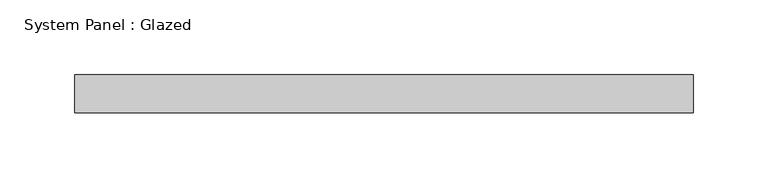
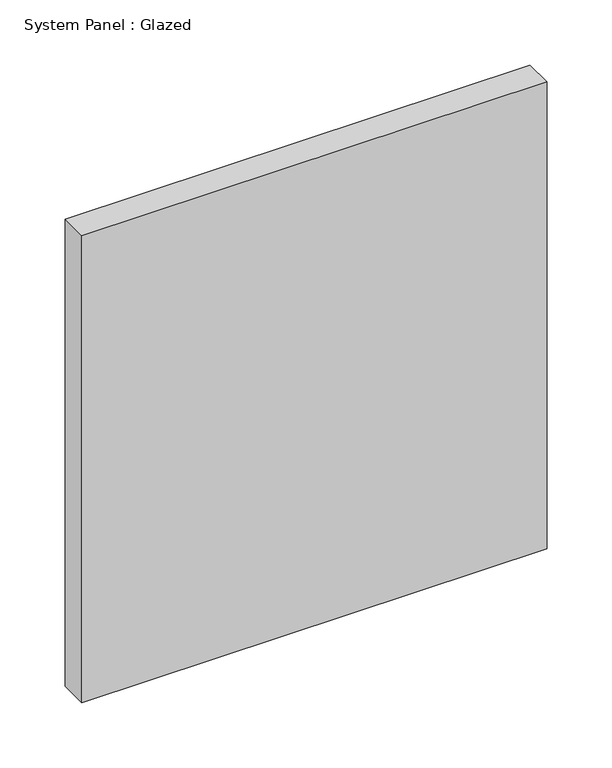
"""IFC4 building model written with IfcOpenShell, lengths in millimetres: plate geometry, System Panel : Glazed."""

from ifc_helpers import new_model, si_unit, origin, origin_with_axes, place, context, project, spatial, polyline, outline, extrude, source, transform, mapped, element, save


def system_panel_glazed_ee3fb3da(model_context):
    return source(origin(), model_context, "Body", "SweptSolid", [
        extrude(outline(polyline([(206.375, 19.05), (-206.375, 19.05), (-206.375, 44.45), (206.375, 44.45), (206.375, 19.05)])), origin_with_axes(), (0.0, 0.0, 1.0), 438.15),
    ])


if __name__ == "__main__":
    model = new_model("IFC4")
    model_context = context("Model", 3, world=origin())
    ifc_project = project(units=[si_unit("LENGTHUNIT", "METRE", prefix="MILLI")], contexts=[model_context])
    site = spatial("IfcSite", under=ifc_project)
    building = spatial("IfcBuilding", under=site)
    placement = place(None, origin())
    system_panel_glazed_shape = system_panel_glazed_ee3fb3da(model_context)
    element("IfcPlate", 1, ObjectType="System Panel : Glazed", at=placement, inside=building, context=model_context, shape_type="MappedRepresentation", body=[
        mapped(system_panel_glazed_shape, transform((0.0, 0.0, 0.0), x_axis=(1.0, 0.0, 0.0), y_axis=(0.0, 1.0, 0.0), z_axis=(0.0, 0.0, 1.0))),
    ])
    save(model, "model.ifc")

# Revit data of these elements
# Type "System Panel : Glazed"
#   Construction Type Id = "GSP4R"
#   Analytic Construction = "1/8 in Pilkington single glazing"
#   Visual Light Transmittance = 0.9
#   Solar Heat Gain Coefficient = 0.86
#   Heat Transfer Coefficient (U) = 1.18115 BTU/(h·ft²·°F)
#   Define Thermal Properties by = 1
# Element 1 (IfcPlate, "System Panel : Glazed")
#   Materials on its faces: "Glass"
# Materials
#   "Glass": class "Glass", colour RGB 0 128 192, transparency 0.75, Description = "Soda Lime Glass", Cost = 0
